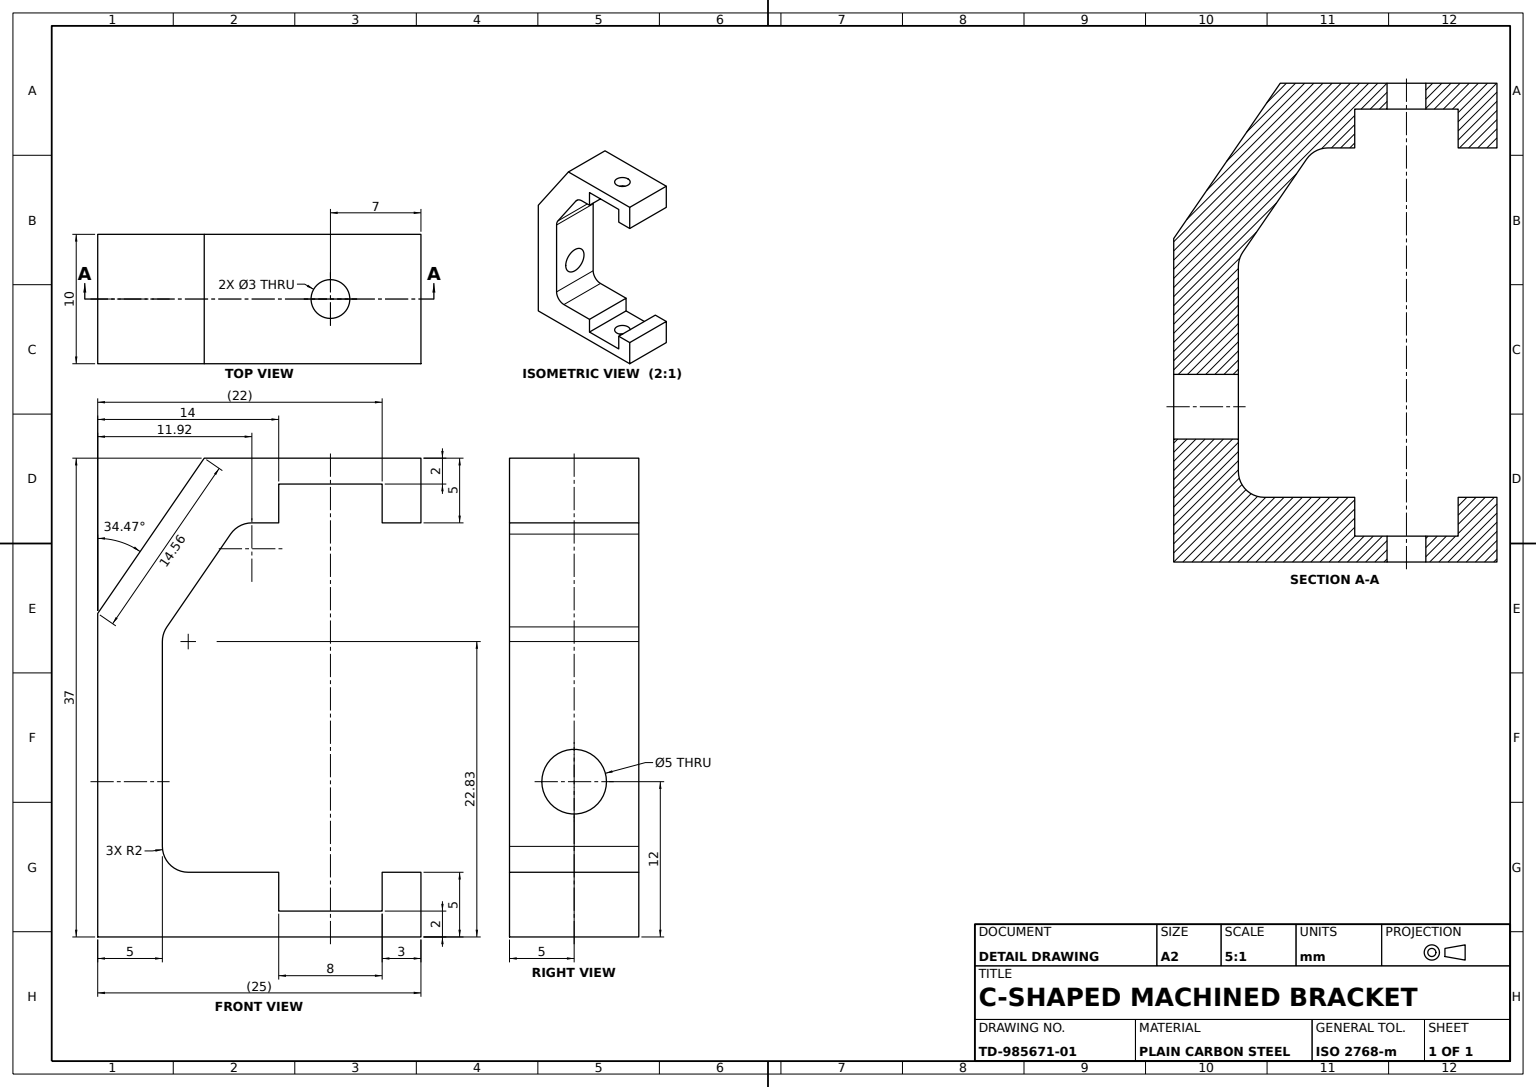
from build123d import *

# Parameters (mm, degrees)
C_BRACKET_BODY_DEPTH      = 5
WEB_HOLE_SKETCH_R         = 2.5
WEB_HOLE_DEPTH            = 10
FLANGE_HOLE_SKETCH_R      = 1.5
FLANGE_THROUGH_HOLE_DEPTH = 51


with BuildPart() as part:
    # Bracket Profile Sketch → C Bracket Body (new, symmetric)
    with BuildSketch(Plane.XY):
        with BuildLine():
            Line((0, 0), (0, 25))
            Line((0, 25), (8.238636364, 37))
            Line((8.238636364, 37), (25, 37))
            Line((25, 37), (25, 32))
            Line((25, 32), (22, 32))
            Line((22, 32), (22, 35))
            Line((22, 35), (14, 35))
            Line((14, 35), (14, 32))
            Line((14, 32), (11.923724939, 32))
            ThreePointArc((11.923724939, 32), (10.992058242, 31.769744944), (10.274912513, 31.131997167))
            Line((10.274912513, 31.131997167), (5.351187575, 23.960337118))
            ThreePointArc((5.351187575, 23.960337118), (5.08981351, 23.420950764), (5, 22.828339951))
            Line((5, 22.828339951), (5, 7))
            ThreePointArc((5, 7), (5.585786438, 5.585786438), (7, 5))
            Line((7, 5), (14, 5))
            Line((14, 5), (14, 2))
            Line((14, 2), (22, 2))
            Line((22, 2), (22, 5))
            Line((22, 5), (25, 5))
            Line((25, 5), (25, 0))
            Line((25, 0), (0, 0))
        make_face()
    extrude(amount=C_BRACKET_BODY_DEPTH, both=True)

    # Web Hole Sketch → Web Hole (cut)
    with BuildSketch(Plane(origin=(5, 0, 0), x_dir=(0, 0, -1), z_dir=(1, 0, 0))):
        with Locations((0, 12)):
            Circle(WEB_HOLE_SKETCH_R)
    extrude(amount=-WEB_HOLE_DEPTH, mode=Mode.SUBTRACT)

    # Flange Hole Sketch → Flange Through Hole (cut)
    with BuildSketch(Plane(origin=(0, 37, 0), x_dir=(1, 0, 0), z_dir=(0, 1, 0))):
        with Locations(Location((18, 0, 0), (0, 0, 270))):
            Circle(FLANGE_HOLE_SKETCH_R)
    extrude(amount=-FLANGE_THROUGH_HOLE_DEPTH, mode=Mode.SUBTRACT)


solid = part.part
